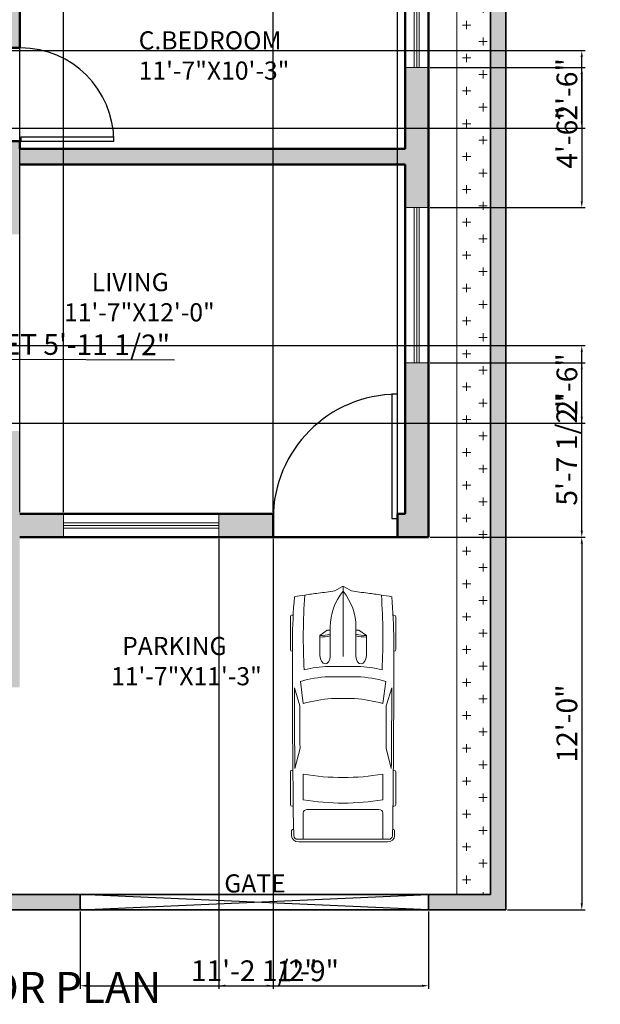
# Model space of a CAD drawing. Units: inches. Extents: x 1369 to 1844, y 2136 to 2743.
# Tile 3 of 4: x 1620 to 1844, y 2136 to 2517. Entities that reach past the tile are written whole.
import ezdxf

# ---------------------------------------------------------------- set-up
doc = ezdxf.new("R2010")
doc.units = ezdxf.units.IN
for name, color, linetype, lineweight in [('A-ANNO-DIMS', 2, 'Continuous', 18), ('A-ANNO-TEXT', 7, 'Continuous', 25), ('A-AREA-IDEN', 7, 'Continuous', 25), ('A-DOOR', 4, 'Continuous', 25), ('A-WALL', 7, 'Continuous', 50), ('C-PRKG-VEHC', 8, 'Continuous', 18), ('C-PROP', 7, 'Continuous', 35), ('L-PLNT', 3, 'Continuous', 18)]:
    doc.layers.add(name, color=color, linetype=linetype, lineweight=lineweight)
for name, color, linetype, lineweight, true_color in [('A-GLAZ', 244, 'Continuous', 20, 0x991b1e), ('A-WALL-PATT', 251, 'Continuous', 13, 0x636466), ('C-PROP-PATT', 251, 'Continuous', 13, 0x636466), ('L-GATE', 244, 'Continuous', 25, 0x991b1e), ('L-PLNT-PATT', 116, 'Continuous', 13, 0x136734)]:
    doc.layers.add(name, color=color, linetype=linetype, lineweight=lineweight, true_color=true_color)
doc.styles.get("Standard").update_dxf_attribs({"font": 'arial.ttf'})
doc.dimstyles.new('ISO-25', dxfattribs={"dimtxt": 8, "dimasz": 2.5, "dimexe": 1.25, "dimexo": 0.625, "dimtad": 1, "dimlunit": 3, "dimtxsty": 'Standard', "dimcen": 2.5, "dimadec": 0, "dimazin": 0, "dimtfac": 1, "dimtmove": 0, "dimatfit": 3, "dimfxl": 1, "dimarcsym": 0})

# ---------------------------------------------------------------- blocks, each defined once
blk = doc.blocks.new('*U2')
for p, q in [((0, 0), (0, -6)), ((-40, 0), (-40, -6))]:
    blk.add_line(p, q)
blk.add_lwpolyline([(0, 0), (0, 40), (-1.75, 40), (-1.75, 0)], close=True)
blk.add_arc((0, 0), 40, 90, 180)
blk = doc.blocks.new('*U11')
for p, q in [((21.1, 37.41), (21.1, 36.83)), ((46.55, 38.89), (22.35, 38.89)), ((47.8, 37.39), (47.8, 37.41)), ((135.45, 37.07), (135.45, 37.41)), ((136.7, 38.89), (160.9, 38.89)), ((162.15, 37.41), (162.15, 36.77)), ((70.03, 31.54), (86.41, 29.35)), ((87.99, 31.87), (74.76, 35.92)), ((134.31, 35.6), (119.29, 31.78)), ((138.42, 29.35), (157.25, 29.35)), ((186.47, 29.35), (167.01, 29.35)), ((186.47, -33.5), (186.47, 33.5)), ((188.4, -32.76), (188.4, 32.76)), ((164.52, 26.39), (164.52, -26.39)), ((32.27, 11.63), (36.13, 17.17)), ((36.13, 17.17), (50.94, 17.17)), ((29.77, 9.51), (51.68, 9.51)), ((32.12, 9.51), (32.12, 11.15)), ((58.92, -10.77), (58.92, 10.77)), ((66.55, -10.53), (66.55, 10.53)), ((82.74, 8.5), (82.74, -8.5)), ((186.47, -10.53), (186.47, 10.53)), ((3.27, 6.13), (0.1, 0.41)), ((0, 0), (51.68, 0)), ((0.1, -0.41), (3.27, -6.13)), ((29.77, -9.51), (51.68, -9.51)), ((32.12, -9.51), (32.12, -11.15)), ((32.27, -11.63), (36.13, -17.17)), ((36.13, -17.17), (50.94, -17.17)), ((86.41, -29.35), (70.03, -31.54)), ((87.99, -31.87), (74.76, -35.92)), ((134.31, -35.6), (119.29, -31.78)), ((157.25, -29.35), (138.42, -29.35)), ((167.01, -29.35), (186.47, -29.35)), ((21.1, -37.41), (21.1, -36.83)), ((46.55, -38.89), (22.35, -38.89)), ((47.8, -37.39), (47.8, -37.41)), ((135.45, -37.07), (135.45, -37.41)), ((136.7, -38.89), (160.9, -38.89)), ((162.15, -37.41), (162.15, -36.77))]:
    blk.add_line(p, q)
for centre, major_axis, ratio, start_param, end_param in [((41.19, -490.86), (0, 528.23), 0.842304, 0.00281, 0.075598), ((22.35, 37.41), (0, -1.48), 0.842304, 3.141593, 4.712389), ((64.48, -10555.62), (0, 10593.03), 0.842304, -0.013397, 0.002797), ((46.55, 37.41), (0, 1.48), 0.842304, -1.570796, 0), ((136.7, 37.41), (0, -1.48), 0.842304, 3.141593, 4.712389), ((160.9, 37.41), (0, 1.48), 0.842304, -1.570796, 0), ((180.63, 35.84), (0, 2.22), 0.842304, -0.013017, 1.249894), ((64.48, -10556.36), (0, 10595.31), 0.842304, -0.013397, -0.013017), ((183.98, 33.5), (0, -2.96), 0.842304, 1.570796, 3.128196), ((183.98, 32.76), (0, -5.25), 0.842304, 1.570796, 3.128196), ((266.03, -27.52), (0, 313.31), 0.842304, 1.367076, 1.39176), ((37.47, -593.96), (0, -623.33), 0.842304, 3.096046, 3.200911), ((135.29, 5.39), (0, 81.77), 0.842304, 1.245306, 1.50788), ((64.48, -10555.62), (0, -10591.55), 0.842304, 3.133765, 3.140441), ((149.6, 2.8), (0, -79.58), 0.842304, 4.372215, 4.640744), ((95.79, -3666.35), (0, -3698.24), 0.842304, 3.134049, 3.144098), ((17.08, 0), (0, 147.02), 0.842304, 4.511394, 4.913384), ((35.91, 0), (0, 147.02), 0.842304, 4.511394, 4.913384), ((167.01, 26.39), (0, 2.96), 0.842304, 0, 1.570796), ((259.18, -27.52), (0, -305.3), 0.842304, 4.528606, 4.561838), ((134.4, 5.39), (0, -89.78), 0.842304, 4.449482, 4.652344), ((-204.49, 52.4), (0, -250.96), 0.842304, 1.385369, 1.434372), ((13.04, 17.01), (0, 27.42), 0.842304, 4.435146, 4.718221), ((14.2, 17.01), (0, 27.42), 0.842304, 4.435146, 4.718221), ((50.79, 13.34), (6.34, -0.36), 0.603834, -1.395552, 1.581315), ((29.77, -46.66), (0, 56.17), 0.842304, 0, 0.590319), ((32.75, 11.15), (0, 0.74), 0.842304, 0.879714, 1.570796), ((0.62, 0), (0, -0.74), 0.842304, 4.131459, 5.293319), ((-204.49, -52.4), (0, 250.96), 0.842304, -1.434372, -1.385369), ((29.77, 46.66), (0, 56.17), 0.842304, 2.551274, 3.141593), ((32.75, -11.15), (0, -0.74), 0.842304, 4.712389, 5.403472), ((13.04, -17.01), (0, -27.42), 0.842304, 1.564964, 1.848039), ((14.2, -17.01), (0, -27.42), 0.842304, 1.564964, 1.848039), ((134.4, -5.39), (0, -89.78), 0.842304, -1.510751, -1.307889), ((135.29, -5.39), (0, -81.77), 0.842304, -1.50788, -1.245306), ((149.6, -2.8), (0, -79.58), 0.842304, -1.499151, -1.230623), ((259.18, 27.52), (0, 305.3), 0.842304, 1.721348, 1.754579), ((266.03, 27.52), (0, 313.31), 0.842304, 1.749832, 1.774517), ((37.47, 593.96), (0, -623.33), 0.842304, -0.059319, 0.045547), ((167.01, -26.39), (0, -2.96), 0.842304, 4.712389, 6.283185), ((41.19, 490.86), (0, -528.23), 0.842304, -0.075598, -0.00281), ((64.48, 10555.62), (0, -10591.55), 0.842304, 0.001152, 0.007828), ((95.79, 3666.35), (0, -3698.24), 0.842304, -0.002505, 0.007544), ((183.98, -33.5), (0, 2.96), 0.842304, 3.15499, 4.712389), ((183.98, -32.76), (0, -5.25), 0.842304, 0.013397, 1.570796), ((22.35, -37.41), (0, 1.48), 0.842304, 1.570796, 3.141593), ((64.48, 10555.62), (0, 10593.03), 0.842304, 3.138796, 3.15499), ((46.55, -37.41), (0, -1.48), 0.842304, 0, 1.570796), ((136.7, -37.41), (0, -1.48), 0.842304, -1.570796, 0), ((160.9, -37.41), (0, 1.48), 0.842304, 3.141593, 4.712389), ((180.63, -35.84), (0, -2.22), 0.842304, -1.249894, 0.013017), ((64.48, 10556.36), (0, 10595.31), 0.842304, 3.15461, 3.15499)]:
    blk.add_ellipse(centre, major_axis=major_axis, ratio=ratio, start_param=start_param, end_param=end_param)
at = {"extrusion": (0, 0, -1)}
blk.add_ellipse((50.79, -13.34), major_axis=(6.34, 0.36), ratio=0.603834, start_param=-1.395552, end_param=1.581315, dxfattribs=at)
blk = doc.blocks.new('WIN-60IN')
for p, q in [((3.5, 0), (3.5, 60)), ((4.5, 0), (4.5, 60)), ((5.5, 0), (5.5, 60))]:
    blk.add_line(p, q)
blk.add_lwpolyline([(0, 60), (9, 60), (9, 0), (0, 0)], close=True)
blk = doc.blocks.new('*D24')
at = {"layer": 'A-ANNO-DIMS', "color": 0, "lineweight": -2, "transparency": 16777216}
for p, q in [((1491.47, 2396.04), (1491.42, 2384.71)), ((1562.89, 2395.76), (1562.84, 2384.42)), ((1493.93, 2385.95), (1560.35, 2385.68)), ((1562.85, 2385.67), (1679.38, 2385.22))]:
    blk.add_line(p, q, dxfattribs=at)
at = {"layer": 'A-ANNO-DIMS', "color": 0, "transparency": 16777216}
for points in [[(1493.93, 2386.36), (1493.93, 2385.53), (1491.43, 2385.96)], [(1560.35, 2386.1), (1560.35, 2385.27), (1562.85, 2385.67)]]:
    blk.add_solid(points, dxfattribs=at)
at = {"layer": 'Defpoints', "color": 0, "transparency": 16777216}
for p in [(1491.47, 2396.67), (1562.89, 2396.39), (1562.85, 2385.67)]:
    blk.add_point(p, dxfattribs=at)
at = {"layer": 'A-ANNO-DIMS', "color": 0, "transparency": 16777216, "insert": (1622.38, 2390.2), "char_height": 8, "attachment_point": 5, "rotation": 359.7742}
blk.add_mtext('DINING SET 5\'-11 1/2"', dxfattribs=at)
blk = doc.blocks.new('*D33')
at = {"layer": 'A-ANNO-DIMS', "color": 0, "lineweight": -2, "transparency": 16777216}
for p, q in [((1778.14, 2498.26), (1838.06, 2498.26)), ((1836.81, 2495.76), (1836.81, 2446.57)), ((1778.14, 2444.07), (1838.06, 2444.07))]:
    blk.add_line(p, q, dxfattribs=at)
at = {"layer": 'A-ANNO-DIMS', "color": 0, "transparency": 16777216}
for points in [[(1836.39, 2495.76), (1837.23, 2495.76), (1836.81, 2498.26)], [(1836.39, 2446.57), (1837.23, 2446.57), (1836.81, 2444.07)]]:
    blk.add_solid(points, dxfattribs=at)
at = {"layer": 'Defpoints', "color": 0, "transparency": 16777216}
for p in [(1777.51, 2498.26), (1777.51, 2444.07), (1836.81, 2444.07)]:
    blk.add_point(p, dxfattribs=at)
at = {"layer": 'A-ANNO-DIMS', "color": 0, "transparency": 16777216, "insert": (1832.1, 2471.16), "char_height": 8, "attachment_point": 5, "rotation": 90}
blk.add_mtext('4\'-6"', dxfattribs=at)
blk = doc.blocks.new('*D34')
at = {"layer": 'A-ANNO-DIMS', "color": 0, "lineweight": -2, "transparency": 16777216}
for p, q in [((1778.14, 2384.07), (1838.06, 2384.07)), ((1836.81, 2319.26), (1836.81, 2381.57)), ((1778.14, 2316.76), (1838.06, 2316.76))]:
    blk.add_line(p, q, dxfattribs=at)
at = {"layer": 'A-ANNO-DIMS', "color": 0, "transparency": 16777216}
for points in [[(1836.39, 2381.57), (1837.23, 2381.57), (1836.81, 2384.07)], [(1836.39, 2319.26), (1837.23, 2319.26), (1836.81, 2316.76)]]:
    blk.add_solid(points, dxfattribs=at)
at = {"layer": 'Defpoints', "color": 0, "transparency": 16777216}
for p in [(1777.51, 2384.07), (1836.81, 2384.07), (1777.51, 2316.76)]:
    blk.add_point(p, dxfattribs=at)
at = {"layer": 'A-ANNO-DIMS', "color": 0, "transparency": 16777216, "insert": (1832.05, 2350.41), "char_height": 8, "attachment_point": 5, "rotation": 90}
blk.add_mtext('5\'-7 1/2"', dxfattribs=at)
blk = doc.blocks.new('*D35')
at = {"layer": 'A-ANNO-DIMS', "color": 0, "lineweight": -2, "transparency": 16777216}
for p, q in [((1778.14, 2316.76), (1838.06, 2316.76)), ((1836.81, 2314.26), (1836.81, 2175.26)), ((1808.14, 2172.76), (1838.06, 2172.76))]:
    blk.add_line(p, q, dxfattribs=at)
at = {"layer": 'A-ANNO-DIMS', "color": 0, "transparency": 16777216}
for points in [[(1836.39, 2314.26), (1837.23, 2314.26), (1836.81, 2316.76)], [(1836.39, 2175.26), (1837.23, 2175.26), (1836.81, 2172.76)]]:
    blk.add_solid(points, dxfattribs=at)
at = {"layer": 'Defpoints', "color": 0, "transparency": 16777216}
for p in [(1777.51, 2316.76), (1807.51, 2172.76), (1836.81, 2172.76)]:
    blk.add_point(p, dxfattribs=at)
at = {"layer": 'A-ANNO-DIMS', "color": 0, "transparency": 16777216, "insert": (1832.1, 2244.76), "char_height": 8, "attachment_point": 5, "rotation": 90}
blk.add_mtext('12\'-0"', dxfattribs=at)
blk = doc.blocks.new('*D45')
at = {"layer": 'A-ANNO-DIMS', "color": 0, "lineweight": -2, "transparency": 16777216}
for p, q in [((1619.51, 2326.38), (1619.51, 2734.31)), ((1622.01, 2733.06), (1634, 2733.06)), ((1636.5, 2326.38), (1636.5, 2734.31)), ((1636.5, 2733.06), (1660.77, 2733.06))]:
    blk.add_line(p, q, dxfattribs=at)
at = {"layer": 'A-ANNO-DIMS', "color": 0, "transparency": 16777216}
for points in [[(1622.01, 2733.47), (1622.01, 2732.64), (1619.51, 2733.06)], [(1634, 2733.47), (1634, 2732.64), (1636.5, 2733.06)]]:
    blk.add_solid(points, dxfattribs=at)
at = {"layer": 'Defpoints', "color": 0, "transparency": 16777216}
for p in [(1636.5, 2733.06), (1619.51, 2325.76), (1636.5, 2325.76)]:
    blk.add_point(p, dxfattribs=at)
at = {"layer": 'A-ANNO-DIMS', "color": 0, "transparency": 16777216, "insert": (1649.88, 2737.77), "char_height": 8, "attachment_point": 5}
blk.add_mtext('1\'-5"', dxfattribs=at)
blk = doc.blocks.new('*D46')
at = {"layer": 'A-ANNO-DIMS', "color": 0, "lineweight": -2, "transparency": 16777216}
for p, q in [((1717.51, 2326.38), (1717.51, 2734.31)), ((1720.01, 2733.06), (1763.01, 2733.06)), ((1765.51, 2326.38), (1765.51, 2734.31))]:
    blk.add_line(p, q, dxfattribs=at)
at = {"layer": 'A-ANNO-DIMS', "color": 0, "transparency": 16777216}
for points in [[(1720.01, 2733.47), (1720.01, 2732.64), (1717.51, 2733.06)], [(1763.01, 2733.47), (1763.01, 2732.64), (1765.51, 2733.06)]]:
    blk.add_solid(points, dxfattribs=at)
at = {"layer": 'Defpoints', "color": 0, "transparency": 16777216}
for p in [(1765.51, 2733.06), (1717.51, 2325.76), (1765.51, 2325.76)]:
    blk.add_point(p, dxfattribs=at)
at = {"layer": 'A-ANNO-DIMS', "color": 0, "transparency": 16777216, "insert": (1741.51, 2737.77), "char_height": 8, "attachment_point": 5}
blk.add_mtext('4\'-0"', dxfattribs=at)
blk = doc.blocks.new('*D47')
at = {"layer": 'A-ANNO-DIMS', "color": 0, "lineweight": -2, "transparency": 16777216}
for p, q in [((1696.5, 2316.13), (1696.5, 2142.21)), ((1717.51, 2316.13), (1717.51, 2142.21)), ((1699, 2143.46), (1715.01, 2143.46)), ((1717.51, 2143.46), (1741.77, 2143.46))]:
    blk.add_line(p, q, dxfattribs=at)
at = {"layer": 'A-ANNO-DIMS', "color": 0, "transparency": 16777216}
for points in [[(1699, 2143.87), (1699, 2143.04), (1696.5, 2143.46)], [(1715.01, 2143.87), (1715.01, 2143.04), (1717.51, 2143.46)]]:
    blk.add_solid(points, dxfattribs=at)
at = {"layer": 'Defpoints', "color": 0, "transparency": 16777216}
for p in [(1696.5, 2316.76), (1717.51, 2316.76), (1717.51, 2143.46)]:
    blk.add_point(p, dxfattribs=at)
at = {"layer": 'A-ANNO-DIMS', "color": 0, "transparency": 16777216, "insert": (1730.89, 2148.17), "char_height": 8, "attachment_point": 5}
blk.add_mtext('1\'-9"', dxfattribs=at)
blk = doc.blocks.new('*D48')
at = {"layer": 'A-ANNO-DIMS', "color": 0, "lineweight": -2, "transparency": 16777216}
for p, q in [((1642.88, 2172.13), (1642.88, 2142.21)), ((1777.51, 2172.13), (1777.51, 2142.21)), ((1645.38, 2143.46), (1775.01, 2143.46))]:
    blk.add_line(p, q, dxfattribs=at)
at = {"layer": 'A-ANNO-DIMS', "color": 0, "transparency": 16777216}
for points in [[(1645.38, 2143.87), (1645.38, 2143.04), (1642.88, 2143.46)], [(1775.01, 2143.87), (1775.01, 2143.04), (1777.51, 2143.46)]]:
    blk.add_solid(points, dxfattribs=at)
at = {"layer": 'Defpoints', "color": 0, "transparency": 16777216}
for p in [(1642.88, 2172.76), (1777.51, 2172.76), (1777.51, 2143.46)]:
    blk.add_point(p, dxfattribs=at)
at = {"layer": 'A-ANNO-DIMS', "color": 0, "transparency": 16777216, "insert": (1710.2, 2148.22), "char_height": 8, "attachment_point": 5}
blk.add_mtext('11\'-2 1/2"', dxfattribs=at)
blk = doc.blocks.new('*D51')
at = {"layer": 'A-ANNO-DIMS', "color": 0, "lineweight": -2, "transparency": 16777216}
for p, q in [((1561.14, 2504.76), (1838.06, 2504.76)), ((1836.81, 2477.26), (1836.81, 2502.26)), ((1561.14, 2474.76), (1838.06, 2474.76))]:
    blk.add_line(p, q, dxfattribs=at)
at = {"layer": 'A-ANNO-DIMS', "color": 0, "transparency": 16777216}
for points in [[(1836.39, 2502.26), (1837.23, 2502.26), (1836.81, 2504.76)], [(1836.39, 2477.26), (1837.23, 2477.26), (1836.81, 2474.76)]]:
    blk.add_solid(points, dxfattribs=at)
at = {"layer": 'Defpoints', "color": 0, "transparency": 16777216}
for p in [(1560.51, 2504.76), (1836.81, 2504.76), (1560.51, 2474.76)]:
    blk.add_point(p, dxfattribs=at)
at = {"layer": 'A-ANNO-DIMS', "color": 0, "transparency": 16777216, "insert": (1832.1, 2489.76), "char_height": 8, "attachment_point": 5, "rotation": 90}
blk.add_mtext('2\'-6"', dxfattribs=at)
blk = doc.blocks.new('*D52')
at = {"layer": 'A-ANNO-DIMS', "color": 0, "lineweight": -2, "transparency": 16777216}
for p, q in [((1472.14, 2390.76), (1838.06, 2390.76)), ((1836.81, 2363.26), (1836.81, 2388.26)), ((1472.14, 2360.76), (1838.06, 2360.76))]:
    blk.add_line(p, q, dxfattribs=at)
at = {"layer": 'A-ANNO-DIMS', "color": 0, "transparency": 16777216}
for points in [[(1836.39, 2388.26), (1837.23, 2388.26), (1836.81, 2390.76)], [(1836.39, 2363.26), (1837.23, 2363.26), (1836.81, 2360.76)]]:
    blk.add_solid(points, dxfattribs=at)
at = {"layer": 'Defpoints', "color": 0, "transparency": 16777216}
for p in [(1471.51, 2390.76), (1836.81, 2390.76), (1471.51, 2360.76)]:
    blk.add_point(p, dxfattribs=at)
at = {"layer": 'A-ANNO-DIMS', "color": 0, "transparency": 16777216, "insert": (1832.1, 2375.76), "char_height": 8, "attachment_point": 5, "rotation": 90}
blk.add_mtext('2\'-6"', dxfattribs=at)

msp = doc.modelspace()

# ---------------------------------------------------------------- hatches: boundary and pattern name
at = {"layer": 'A-WALL-PATT'}
h = msp.add_hatch(color=256, dxfattribs=at)
h.dxf.hatch_style = 1
h.paths.add_polyline_path([(1619.511, 2460.756), (1768.511, 2460.756), (1768.511, 2444.065), (1777.511, 2444.065), (1777.511, 2498.256), (1768.511, 2498.256), (1768.511, 2466.756), (1619.511, 2466.756), (1619.511, 2469.756), (1614.511, 2469.756), (1613.511, 2469.756), (1613.511, 2433.756), (1619.511, 2433.756)])
h.paths.add_polyline_path([(1480.511, 2453.756), (1560.511, 2453.756), (1560.511, 2474.756), (1556.011, 2474.756), (1554.511, 2474.756), (1554.511, 2459.756), (1462.511, 2459.756), (1462.511, 2473.256), (1453.511, 2473.256), (1453.511, 2453.756), (1471.511, 2453.756), (1471.511, 2390.756), (1480.511, 2390.756)])
h.paths.add_polyline_path([(1574.511, 2513.156), (1574.511, 2513.756), (1462.511, 2513.756), (1462.511, 2551.882), (1453.511, 2551.882), (1453.511, 2494.256), (1462.511, 2494.256), (1462.511, 2507.756), (1554.511, 2507.756), (1554.511, 2504.756), (1556.011, 2504.756), (1560.511, 2504.756), (1560.511, 2507.756), (1574.511, 2507.756)])
h.paths.add_polyline_path([(1462.511, 2351.756), (1480.511, 2351.756), (1480.511, 2357.756), (1480.511, 2360.756), (1476.011, 2360.756), (1471.511, 2360.756), (1471.511, 2357.756), (1453.511, 2357.756), (1453.511, 2258.756), (1508.011, 2258.756), (1508.011, 2267.756), (1462.511, 2267.756)])
h.paths.add_polyline_path([(1619.511, 2357.756), (1592.511, 2357.756), (1592.511, 2351.756), (1613.511, 2351.756), (1613.511, 2267.756), (1568.011, 2267.756), (1568.011, 2258.756), (1619.511, 2258.756), (1619.511, 2316.756), (1636.503, 2316.756), (1636.503, 2325.756), (1619.511, 2325.756)])
h.paths.add_polyline_path([(1717.511, 2323.956), (1717.511, 2325.756), (1696.503, 2325.756), (1696.503, 2316.756), (1717.511, 2316.756)])
h.paths.add_polyline_path([(1777.511, 2384.065), (1768.511, 2384.065), (1768.511, 2325.756), (1765.511, 2325.756), (1765.511, 2323.956), (1765.511, 2316.756), (1777.511, 2316.756)])
h.paths.add_polyline_path([(1777.511, 2652.756), (1731.511, 2652.756), (1731.511, 2643.756), (1768.511, 2643.756), (1768.511, 2595.756), (1673.511, 2595.756), (1673.511, 2598.756), (1672.011, 2598.756), (1667.511, 2598.756), (1667.511, 2595.756), (1613.511, 2595.756), (1613.511, 2513.756), (1610.511, 2513.756), (1610.511, 2513.156), (1610.511, 2507.756), (1613.511, 2507.756), (1613.511, 2505.756), (1619.511, 2505.756), (1619.511, 2589.756), (1768.511, 2589.756), (1768.511, 2558.256), (1777.511, 2558.256)])
h.paths.add_polyline_path([(1710.511, 2652.756), (1616.643, 2652.756), (1616.643, 2643.756), (1667.511, 2643.756), (1667.511, 2628.756), (1672.011, 2628.756), (1673.511, 2628.756), (1673.511, 2643.756), (1710.511, 2643.756)], flags=17)
h.paths.add_polyline_path([(1556.643, 2652.756), (1453.511, 2652.756), (1453.511, 2611.882), (1462.511, 2611.882), (1462.511, 2643.756), (1556.643, 2643.756)])
at = {"layer": 'C-PROP-PATT'}
h = msp.add_hatch(color=256, dxfattribs=at)
h.dxf.hatch_style = 1
h.paths.add_polyline_path([(1423.511, 2676.756), (1801.511, 2676.756), (1801.511, 2178.756), (1777.511, 2178.756), (1777.511, 2172.756), (1807.511, 2172.756), (1807.511, 2682.756), (1414.511, 2682.756), (1414.511, 2172.756), (1642.884, 2172.756), (1642.884, 2178.756), (1423.511, 2178.756)])
at = {"layer": 'L-PLNT-PATT'}
h = msp.add_hatch(dxfattribs=at)
h.set_pattern_fill('CROSS', color=256)
h.paths.add_polyline_path([(1453.511, 2652.756), (1777.511, 2652.756), (1788.511, 2652.756), (1788.511, 2178.756), (1801.511, 2178.756), (1801.511, 2676.756), (1423.511, 2676.756), (1423.511, 2453.756), (1453.511, 2453.756)])
h.paths.add_polyline_path([(1453.511, 2350.279), (1423.511, 2350.279), (1423.511, 2178.756), (1453.511, 2178.756), (1453.511, 2258.756)], flags=17)

# ---------------------------------------------------------------- linework, layer by layer
at = {"layer": 'A-WALL'}
for p, q in [((1777.511, 2652.756), (1777.511, 2316.756)), ((1619.511, 2589.756), (1619.511, 2505.756)), ((1768.511, 2589.756), (1768.511, 2466.756)), ((1619.511, 2505.756), (1613.511, 2505.756)), ((1619.511, 2469.756), (1613.511, 2469.756)), ((1619.511, 2469.756), (1619.511, 2466.756)), ((1619.511, 2466.756), (1768.511, 2466.756)), ((1619.511, 2460.756), (1768.511, 2460.756)), ((1768.511, 2460.756), (1768.511, 2325.756)), ((1619.511, 2325.756), (1717.511, 2325.756)), ((1717.511, 2325.756), (1717.511, 2316.756)), ((1765.511, 2325.756), (1765.511, 2316.756)), ((1765.511, 2325.756), (1768.511, 2325.756)), ((1619.511, 2316.756), (1777.511, 2316.756))]:
    msp.add_line(p, q, dxfattribs=at)
at = {"layer": 'C-PROP'}
for p, q in [((1807.511, 2682.756), (1807.511, 2172.756)), ((1801.511, 2676.756), (1801.511, 2178.756)), ((1423.511, 2178.756), (1801.511, 2178.756)), ((1642.884, 2178.756), (1642.884, 2172.756)), ((1777.511, 2178.756), (1777.511, 2172.756)), ((1414.511, 2172.756), (1807.511, 2172.756))]:
    msp.add_line(p, q, dxfattribs=at)
at = {"layer": 'L-GATE'}
for p, q in [((1642.884, 2172.756), (1777.511, 2178.756)), ((1777.511, 2172.756), (1642.884, 2178.756))]:
    msp.add_line(p, q, dxfattribs=at)
at = {"layer": 'L-PLNT'}
msp.add_line((1788.511, 2652.756), (1788.511, 2178.756), dxfattribs=at)

# ---------------------------------------------------------------- block references
at = {"layer": 'A-DOOR', "xscale": 0.9, "yscale": 0.9, "zscale": 0.9, "rotation": 270}
msp.add_blockref('*U2', (1619.911, 2469.756), dxfattribs=at)
at = {"layer": 'A-DOOR', "xscale": 1.199999999999994, "yscale": 1.199999999999994, "zscale": 1.199999999999994}
msp.add_blockref('*U2', (1765.511, 2323.956), dxfattribs=at)
at = {"layer": 'A-GLAZ'}
for p in [(1768.511, 2498.256), (1768.511, 2384.065)]:
    msp.add_blockref('WIN-60IN', p, dxfattribs=at)
at = {"layer": 'A-GLAZ', "rotation": 269.9999999999998}
msp.add_blockref('WIN-60IN', (1636.503, 2325.756), dxfattribs=at)
at = {"layer": 'C-PRKG-VEHC', "xscale": 0.5238111194664629, "yscale": 0.5238111194664629, "zscale": 0.5238111194664629, "rotation": 270}
msp.add_blockref('*U11', (1744.536, 2297.716), dxfattribs=at)

# ---------------------------------------------------------------- texts
at = {"layer": 'A-ANNO-TEXT', "attachment_point": 1}
for s, width, insert, char_height in [('GATE', 27.18559, (1698.617, 2186.495), 7), ('GROUND FLOOR PLAN', 194.0265, (1504.541, 2148.798), 12)]:
    msp.add_mtext_dynamic_manual_height_columns(s, width=width, gutter_width=12.5, heights=[0], dxfattribs=dict(at, insert=insert, char_height=char_height))
at = {"layer": 'A-AREA-IDEN', "char_height": 7, "attachment_point": 1}
for s, width, insert in [('C.BEDROOM    11\'-7"X10\'-3"', 62.44509, (1665.511, 2512.198)), ('     LIVING\\P11\'-7"X12\'-0"', 57.85744, (1636.653, 2418.802)), ('  PARKING\\P11\'-7"X11\'-3"', 57.85744, (1654.842, 2278.21))]:
    msp.add_mtext_dynamic_manual_height_columns(s, width=width, gutter_width=12.5, heights=[0], dxfattribs=dict(at, insert=insert))

# ---------------------------------------------------------------- dimensions: what is measured, and where the dimension line sits
at = {"layer": 'A-ANNO-DIMS'}
for base, p1, p2, picture, middle in [((1636.503, 2733.056), (1619.511, 2325.756), (1636.503, 2325.756), '*D45', (1649.884, 2737.766)), ((1765.511, 2733.056), (1717.511, 2325.756), (1765.511, 2325.756), '*D46', (1741.511, 2737.766)), ((1717.511, 2143.456), (1696.503, 2316.756), (1717.511, 2316.756), '*D47', (1730.893, 2148.166)), ((1777.511, 2143.456), (1642.884, 2172.756), (1777.511, 2172.756), '*D48', (1710.198, 2148.217))]:
    dim = msp.add_linear_dim(base=base, p1=p1, p2=p2, dimstyle='ISO-25', override={"dimdec": 1, "dimlfac": 1, "dimrnd": 0, "dimzin": 1, "dimdsep": 46, "dimlunit": 4, "dimfrac": 2}, dxfattribs=at)
    dim.commit()
    dim.dimension.update_dxf_attribs({"geometry": picture, "text_midpoint": middle})
for base, p1, p2, picture, middle in [((1836.811, 2504.756), (1560.511, 2474.756), (1560.511, 2504.756), '*D51', (1832.102, 2489.756)), ((1836.811, 2444.065), (1777.511, 2498.256), (1777.511, 2444.065), '*D33', (1832.102, 2471.161)), ((1836.811, 2390.756), (1471.511, 2360.756), (1471.511, 2390.756), '*D52', (1832.102, 2375.756)), ((1836.811, 2384.065), (1777.511, 2316.756), (1777.511, 2384.065), '*D34', (1832.05, 2350.411)), ((1836.811, 2172.756), (1777.511, 2316.756), (1807.511, 2172.756), '*D35', (1832.102, 2244.756))]:
    dim = msp.add_linear_dim(base=base, p1=p1, p2=p2, angle=90, dimstyle='ISO-25', override={"dimdec": 1, "dimlfac": 1, "dimrnd": 0, "dimzin": 1, "dimdsep": 46, "dimlunit": 4, "dimfrac": 2}, dxfattribs=at)
    dim.commit()
    dim.dimension.update_dxf_attribs({"geometry": picture, "text_midpoint": middle})
dim = msp.add_linear_dim(base=(1562.848, 2385.674), p1=(1491.47, 2396.669), p2=(1562.89, 2396.387), angle=359.77416, text='DINING SET <>', dimstyle='ISO-25', override={"dimdec": 1, "dimlfac": 1, "dimrnd": 0, "dimzin": 1, "dimdsep": 46, "dimlunit": 4, "dimfrac": 2}, dxfattribs=at)
dim.commit()
dim.dimension.update_dxf_attribs({"geometry": '*D24', "text_midpoint": (1622.384, 2390.201)})

doc.saveas('drawing.dxf')
